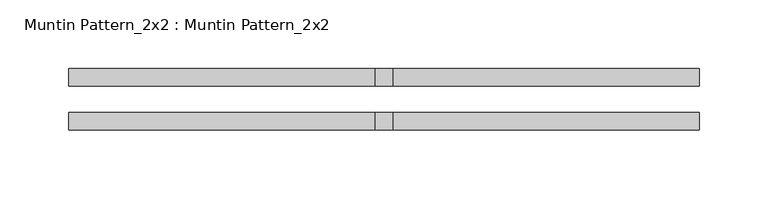
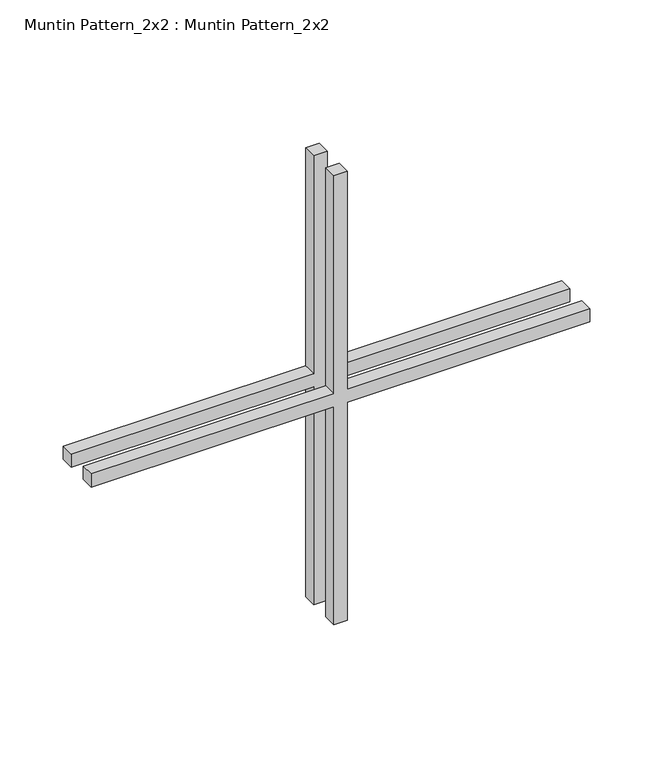
"""IFC4 building model written with IfcOpenShell, lengths in millimetres: proxy geometry, Muntin Pattern_2x2 : Muntin Pattern_2x2."""

from ifc_helpers import new_model, si_unit, frame, origin, place, context, project, spatial, polyline, outline, extrude, source, transform, mapped, element, save


def muntin_pattern_2x2_muntin_pattern_2x2_eba6c5fb(model_context):
    return source(origin(), model_context, "Body", "SweptSolid", [
        extrude(outline(polyline([(223.8375, -6.35), (223.8375, -228.6), (211.1375, -228.6), (211.1375, -6.35), (0.0, -6.35), (0.0, 6.35), (211.1375, 6.35), (211.1375, 228.6), (223.8375, 228.6), (223.8375, 6.35), (434.975, 6.35), (434.975, -6.35), (223.8375, -6.35)])), frame((0.0, 9.525, 0.0), z_axis=(0.0, 1.0, 0.0), x_axis=(0.0, 0.0, 1.0)), (0.0, 0.0, 1.0), 12.7),
        extrude(outline(polyline([(223.8375, -6.35), (223.8375, -228.6), (211.1375, -228.6), (211.1375, -6.35), (0.0, -6.35), (0.0, 6.35), (211.1375, 6.35), (211.1375, 228.6), (223.8375, 228.6), (223.8375, 6.35), (434.975, 6.35), (434.975, -6.35), (223.8375, -6.35)])), frame((0.0, -22.225, 0.0), z_axis=(0.0, 1.0, 0.0), x_axis=(0.0, 0.0, 1.0)), (0.0, 0.0, 1.0), 12.7),
    ])


if __name__ == "__main__":
    model = new_model("IFC4")
    model_context = context("Model", 3, world=origin())
    ifc_project = project(units=[si_unit("LENGTHUNIT", "METRE", prefix="MILLI")], contexts=[model_context])
    site = spatial("IfcSite", under=ifc_project)
    building = spatial("IfcBuilding", under=site)
    placement = place(None, origin())
    muntin_pattern_2x2_muntin_pattern_2x2_shape = muntin_pattern_2x2_muntin_pattern_2x2_eba6c5fb(model_context)
    element("IfcBuildingElementProxy", 1, Name="Muntin Pattern_2x2 : Muntin Pattern_2x2", ObjectType="Muntin Pattern_2x2 : Muntin Pattern_2x2", at=placement, inside=building, context=model_context, shape_type="MappedRepresentation", body=[
        mapped(muntin_pattern_2x2_muntin_pattern_2x2_shape, transform((0.0, 0.0, 0.0), x_axis=(1.0, 0.0, 0.0), y_axis=(0.0, 1.0, 0.0), z_axis=(0.0, 0.0, 1.0))),
    ])
    save(model, "model.ifc")

# Revit data of these elements
# Type "Muntin Pattern_2x2 : Muntin Pattern_2x2"
#   Width [instance default] = 4' - 0"
#   Thickness = 0' - 0 1/2"
#   Height [instance default] = 4' - 0"
#   Distance = 0' - 0 3/4"
#   Interior Material [instance default] = none
#   Exterior Material [instance default] = none
#   Default Elevation = 0
# Element 1 (IfcBuildingElementProxy, "Muntin Pattern_2x2 : Muntin Pattern_2x2")
#   Width = 1' - 6"
#   Height = 1' - 5 1/8"
#   Interior Material = Wood - Stained
#   Exterior Material = Clad - White
#   Materials on its faces: "Clad - White", "Wood - Stained"
# Materials
#   "Clad - White": class "Wood", colour RGB 242 242 238, transparency 0, Cost = 0
#   "Wood - Stained": class "Wood", colour RGB 224 178 126, transparency 0, Cost = 0
